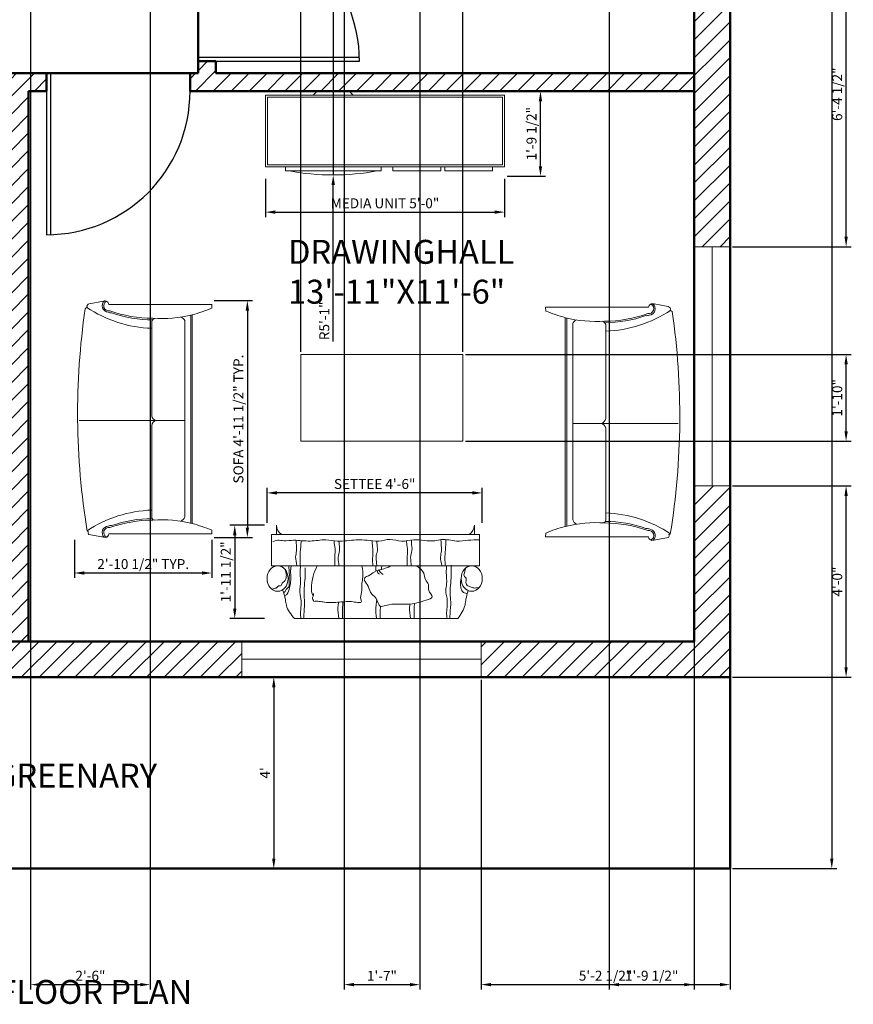
# Model space of a CAD drawing. Units: inches. Extents: x 3887 to 4286, y 884 to 1458.
# Tile 2 of 4: x 4077 to 4286, y 884 to 1131. Entities that reach past the tile are written whole.
import ezdxf

# ---------------------------------------------------------------- set-up
doc = ezdxf.new("R2010")
doc.units = ezdxf.units.IN
for name, color, linetype, lineweight in [('A-ANNO-DIMS', 2, 'Continuous', 18), ('A-ANNO-TEXT', 7, 'Continuous', 25), ('A-AREA-IDEN', 7, 'Continuous', 25), ('A-DOOR', 3, 'Continuous', 25), ('A-FURN', 8, 'Continuous', 18), ('A-GLAZ', 4, 'Continuous', 18), ('A-WALL', 7, 'Continuous', 50), ('A-WALL-PATT', 252, 'Continuous', 13)]:
    doc.layers.add(name, color=color, linetype=linetype, lineweight=lineweight)
doc.styles.get("Standard").update_dxf_attribs({"font": 'arial.ttf'})
doc.dimstyles.new('ISO-25', dxfattribs={"dimtxt": 2.5, "dimasz": 2.5, "dimexe": 1.25, "dimexo": 0.625, "dimtad": 1, "dimdec": 0, "dimlunit": 3, "dimtxsty": 'Standard', "dimcen": 2.5, "dimadec": 0, "dimazin": 0, "dimtfac": 1, "dimtdec": 0, "dimtmove": 0, "dimatfit": 3, "dimfxl": 1, "dimarcsym": 0})

# ---------------------------------------------------------------- blocks, each defined once
blk = doc.blocks.new('A$C69644375')
for p, q in [((1847.6, 919.1), (239.3, 919.1)), ((27.1, 91.8), (27.1, 399)), ((2073.7, 399), (27.1, 399)), ((2073.7, 399), (2073.7, 91.8)), ((2073.7, 91.8), (27.1, 91.8)), ((78.1, 91.8), (78.1, 0)), ((2025.4, 91.8), (2025.4, 0))]:
    blk.add_line(p, q)
for centre, start, end in [((187.1, -0.8), 121.46958, 179.57872), ((1916.5, -0.8), 0.42128, 58.53042)]:
    blk.add_arc(centre, 109, start, end)
at = {"extrusion": (0, 0, -1)}
for centre in [(103.9, 524.8), (2014.8, 524.8)]:
    blk.add_ellipse(centre, major_axis=(0, 125.7), ratio=0.82705, start_param=3.141593, end_param=9.424778, dxfattribs=at)
for points, knots in [([(137.7, 643.7), (147.1, 671.6), (161.1, 717.2), (170.9, 816.6), (209.4, 875.9), (239.3, 919.1)], [21.621392, 21.621392, 21.621392, 21.621392, 109.715225, 164.717522, 317.924576, 317.924576, 317.924576, 317.924576]), ([(318.6, 917.6), (317.6, 889.5), (316, 841.4), (307.9, 766.7), (315.9, 694.6), (316.1, 610.2), (302.9, 510.5), (305.2, 435.5), (306.5, 392.7)], [0, 0, 0, 0, 84.237495, 144.472456, 224.70795, 300.836536, 397.332321, 525.548945, 525.548945, 525.548945, 525.548945]), ([(346.9, 919.1), (349.1, 898.5), (352.8, 861.9), (344.6, 797.5), (341.7, 724.7), (365.6, 649.2), (342.5, 562.7), (358.6, 480.7), (352.8, 419.4), (350.6, 396.7)], [2.477757, 2.477757, 2.477757, 2.477757, 64.233403, 112.481299, 196.623447, 281.619849, 342.25328, 458.518645, 526.75141, 526.75141, 526.75141, 526.75141]), ([(671.2, 917.6), (671.9, 886.8), (673.2, 837.4), (668.4, 788.2), (667.2, 769.6)], [0, 0, 0, 0, 92.15571, 148.118503, 148.118503, 148.118503, 148.118503]), ([(707.2, 917.6), (712.9, 880.1), (720.1, 832.7), (712.8, 785.9), (711.3, 776.2)], [0, 0, 0, 0, 112.475377, 141.942796, 141.942796, 141.942796, 141.942796]), ([(1003.7, 917.6), (1004.5, 886.8), (1005.5, 846.8), (1002.6, 807.1), (1001.9, 798)], [0, 0, 0, 0, 92.15571, 119.67693, 119.67693, 119.67693, 119.67693]), ([(1039.8, 917.6), (1045.5, 880.1), (1054.2, 822.3), (1040.4, 760.3), (1039.1, 735.1), (1038.9, 730)], [0, 0, 0, 0, 112.475377, 173.108808, 188.403296, 188.403296, 188.403296, 188.403296]), ([(1376.3, 917.6), (1377.1, 886.8), (1378.5, 832.2), (1372.6, 777.9), (1371.6, 754.1)], [0, 0, 0, 0, 92.15571, 163.700074, 163.700074, 163.700074, 163.700074]), ([(1412.4, 917.6), (1418.1, 880.1), (1426.2, 826.7), (1415.9, 773.9), (1413.8, 758.1)], [0, 0, 0, 0, 112.475377, 160.127407, 160.127407, 160.127407, 160.127407]), ([(1757, 917.6), (1756.1, 889.5), (1754.5, 841.4), (1746.4, 766.7), (1754.3, 694.6), (1754.6, 610.2), (1742.2, 519.8), (1744, 454.1), (1745, 420.7)], [0, 0, 0, 0, 84.237495, 144.472456, 224.70795, 300.836536, 397.332321, 497.501547, 497.501547, 497.501547, 497.501547]), ([(1785.3, 919.1), (1787.5, 898.5), (1791.2, 861.9), (1783, 797.5), (1780.1, 724.7), (1804.1, 649.2), (1780.9, 562.7), (1797, 482), (1791.1, 422), (1789, 400.7)], [2.477757, 2.477757, 2.477757, 2.477757, 64.233403, 112.481299, 196.623447, 281.619849, 342.25328, 458.518645, 522.751997, 522.751997, 522.751997, 522.751997]), ([(1965.1, 635.2), (1954, 667.2), (1937.6, 716.7), (1928.4, 821.8), (1882.5, 878), (1847.6, 919.1)], [8.444588, 8.444588, 8.444588, 8.444588, 109.715225, 164.717522, 319.974725, 319.974725, 319.974725, 319.974725]), ([(1164, 540.9), (1149.2, 559.9), (1117.1, 601.1), (1100.8, 678.6), (1029.2, 716.5), (1023.2, 814.8), (886.4, 762.4), (735.7, 792.7), (603.6, 754.7), (466.8, 709.8), (540.8, 647.1), (520.4, 581.6), (567.2, 534.8), (568.3, 454.9), (616.9, 421.5), (647.1, 400.7)], [0, 0, 0, 0, 72.233047, 156.470492, 218.801185, 304.830125, 357.530882, 582.231345, 763.024758, 827.63193, 899.307199, 955.544862, 1014.704082, 1076.905882, 1178.90147, 1178.90147, 1178.90147, 1178.90147]), ([(1656.8, 749.3), (1639.4, 748.5), (1604.4, 747), (1521.3, 765.5), (1410.9, 759.8), (1291.1, 744.1), (1228, 763.8), (1183.4, 759.1), (1207.7, 711.2), (1178.9, 657), (1189.1, 581.5), (1169.4, 496.1), (1178.3, 438.3), (1184, 400.7)], [0, 0, 0, 0, 52.087932, 104.788603, 253.038902, 385.322741, 449.929867, 466.450206, 494.782313, 563.367144, 651.607113, 712.240498, 824.715876, 824.715876, 824.715876, 824.715876]), ([(1624.8, 400.7), (1639.9, 432.9), (1672.6, 502.7), (1682.2, 608.8), (1680.5, 659), (1668.8, 693.2), (1666.1, 685.2), (1664.8, 681.2)], [0, 0, 0, 0, 107.885542, 233.125089, 289.789384, 298.748781, 307.708142, 307.708142, 307.708142, 307.708142]), ([(1656.8, 749.3), (1664.8, 737.1), (1678.8, 715.8), (1659.5, 691.2), (1660.6, 677.2), (1660.9, 673)], [0, 0, 0, 0, 38.983085, 68.164145, 80.629677, 80.629677, 80.629677, 80.629677]), ([(1944.6, 700.6), (1937.4, 694.7), (1913.3, 671.5), (1899.8, 624.7), (1885.6, 565.8), (1884, 504.8), (1888.2, 447.1), (1882.7, 414), (1881.2, 404.7)], [34.701734, 34.701734, 34.701734, 34.701734, 62.587656, 136.251197, 173.191811, 245.424854, 317.546682, 345.878835, 345.878835, 345.878835, 345.878835]), ([(40, 613), (55.1, 616.5), (81.9, 622.6), (114.8, 602.8), (156.8, 597.6), (164, 555), (153.4, 520), (185.1, 504.2), (175.7, 465.1), (168.2, 441.4), (164.2, 428.7)], [0, 0, 0, 0, 44.256189, 78.489965, 112.723816, 158.407978, 186.455377, 209.121029, 245.181943, 287.01386, 287.01386, 287.01386, 287.01386]), ([(147.5, 674.2), (160.5, 671.6), (192.4, 665.4), (222.4, 596), (211.6, 543), (204.5, 508)], [0, 0, 0, 0, 38.011492, 93.00469, 199.417844, 199.417844, 199.417844, 199.417844]), ([(1955.3, 664.3), (1949.7, 661.6), (1936.7, 652), (1931.5, 625), (1901, 612.3), (1902, 536.8), (1895.8, 472.8), (1903.7, 415.4), (1905.2, 404.7)], [33.002736, 33.002736, 33.002736, 33.002736, 52.087989, 84.391566, 104.42539, 141.366005, 281.602903, 313.906504, 313.906504, 313.906504, 313.906504]), ([(2061.5, 621), (2046.3, 621.9), (2022.8, 623.2), (2009, 591.4), (1977.1, 604.2), (1975, 565.6), (1937.3, 551.2), (1929.2, 512.4), (1928.2, 473.5), (1936, 454), (1941.3, 440.7)], [0, 0, 0, 0, 40.861148, 63.526857, 83.56064, 115.864217, 141.52001, 197.327846, 217.361728, 259.193601, 259.193601, 259.193601, 259.193601]), ([(1160, 532.9), (1159.2, 527.1), (1156.4, 506.9), (1107.3, 497.5), (1058.9, 447.6), (977.8, 435.3), (923.1, 412.5), (900, 401), (896.2, 399)], [0, 0, 0, 0, 16.520339, 57.77249, 124.458333, 225.822378, 290.553607, 303.2098, 303.2098, 303.2098, 303.2098]), ([(1019.7, 436.7), (1016.1, 443.7), (1005.7, 463.3), (987.4, 476.4), (975.7, 484.8)], [0, 0, 0, 0, 23.363259, 65.955745, 65.955745, 65.955745, 65.955745]), ([(364.3, 399), (365.1, 387.6), (368, 350.7), (368.2, 281.6), (358.1, 207.4), (357.5, 158.2), (357.6, 141)], [190.255604, 190.255604, 190.255604, 190.255604, 224.70795, 300.836536, 397.332321, 448.655162, 448.655162, 448.655162, 448.655162]), ([(398.4, 399), (398.5, 398.3), (402.3, 369.2), (417.8, 320.6), (394.6, 235.6), (407, 177.9), (406.8, 140.7)], [194.236029, 194.236029, 194.236029, 194.236029, 196.623447, 281.619849, 342.25328, 454.038772, 454.038772, 454.038772, 454.038772]), ([(698.2, 399), (698.3, 392.9), (700.2, 358.5), (711.7, 313.8), (687.5, 252.5), (694.1, 201.4), (698.1, 160.3), (698.2, 146.5)], [190.129367, 190.129367, 190.129367, 190.129367, 208.421077, 292.658572, 321.828316, 401.96366, 443.368776, 443.368776, 443.368776, 443.368776]), ([(738.4, 399), (737.9, 374.3), (742.3, 323.9), (730.9, 250.8), (742.4, 194.1), (745.1, 162.4), (745.6, 153.4)], [190.836968, 190.836968, 190.836968, 190.836968, 265.264473, 341.498474, 410.083305, 437.099432, 437.099432, 437.099432, 437.099432]), ([(1031.8, 448.8), (1031.5, 456.1), (1030.9, 470.6), (1018.1, 477.4), (1011.7, 480.8)], [0, 0, 0, 0, 20.430573, 40.464424, 40.464424, 40.464424, 40.464424]), ([(1038.7, 399), (1038.9, 392.9), (1040.7, 358.5), (1052.2, 313.8), (1028.1, 252.5), (1034.2, 205), (1037.9, 167.4), (1038.5, 157)], [190.129367, 190.129367, 190.129367, 190.129367, 208.421077, 292.658572, 321.828316, 401.96366, 432.870883, 432.870883, 432.870883, 432.870883]), ([(1078.9, 399), (1078.4, 374.3), (1082.9, 323.9), (1071.4, 250.8), (1082.9, 194.3), (1085.6, 162.7), (1086.2, 153.9)], [190.836968, 190.836968, 190.836968, 190.836968, 265.264473, 341.498474, 410.083305, 436.597925, 436.597925, 436.597925, 436.597925]), ([(1411.4, 399), (1411.5, 392.9), (1413.4, 358.5), (1424.9, 313.8), (1400.7, 252.5), (1406.8, 204.9), (1410.6, 167.2), (1411.1, 156.8)], [190.129367, 190.129367, 190.129367, 190.129367, 208.421077, 292.658572, 321.828316, 401.96366, 433.110807, 433.110807, 433.110807, 433.110807]), ([(1451.6, 399), (1451.1, 374.3), (1455.5, 323.9), (1444.1, 250.8), (1455.6, 194), (1458.3, 162.1), (1458.9, 152.9)], [190.836968, 190.836968, 190.836968, 190.836968, 265.264473, 341.498474, 410.083305, 437.573854, 437.573854, 437.573854, 437.573854]), ([(1790.7, 399), (1791.5, 387.6), (1794.4, 350.7), (1794.6, 281.6), (1785, 210.8), (1784, 165.1), (1784, 151.4)], [190.255604, 190.255604, 190.255604, 190.255604, 224.70795, 300.836536, 397.332321, 438.291577, 438.291577, 438.291577, 438.291577]), ([(1824.8, 399), (1824.9, 398.3), (1828.7, 369.2), (1844.2, 320.6), (1821.7, 238.2), (1832.4, 183), (1833.1, 148.3)], [194.236029, 194.236029, 194.236029, 194.236029, 196.623447, 281.619849, 342.25328, 446.449161, 446.449161, 446.449161, 446.449161]), ([(2061.5, 160.3), (2045.6, 154.9), (2010.3, 143.1), (1941.1, 157.7), (1834.5, 140.2), (1696.7, 167.9), (1552.4, 133.8), (1402, 167.9), (1265.6, 139.7), (1130.5, 145.9), (1019.2, 166.3), (907.6, 126.7), (793, 169.1), (646.4, 126.8), (513.3, 169.9), (375.5, 127.4), (265.2, 167.3), (141, 145.4), (66.1, 144.6), (30.1, 144.2)], [0, 0, 0, 0, 49.560916, 109.795839, 206.041565, 370.514196, 523.244954, 640.061112, 824.76374, 933.020566, 1045.495763, 1158.824136, 1272.152508, 1392.954889, 1601.460588, 1666.685979, 1815.800011, 1932.272164, 2040.52891, 2040.52891, 2040.52891, 2040.52891])]:
    blk.add_open_spline(points, degree=3, knots=knots)
for points in [[(995.1, 436.3), (993.3, 423), (990.5, 409.8), (987.7, 396.7)], [(1047.5, 452.6), (1047.9, 435.3), (1047.9, 418), (1047.8, 400.7)]]:
    blk.add_open_spline(points, degree=3)
blk = doc.blocks.new('A$C73531C16')
for p, q in [((797.3, 883), (797.3, 180.7)), ((797.3, 883), (797.3, 180.7)), ((19.2, 817.1), (1.4, 722.3)), ((19.2, 817.1), (1.4, 722.3)), ((1533.5, 830.9), (1538.9, 821.6)), ((1533.5, 830.9), (1538.9, 821.6)), ((1576, 707.8), (1556.2, 818.7)), ((1576, 707.8), (1556.2, 818.7)), ((23.8, 686), (23.8, 0)), ((23.8, 686), (23.8, 0)), ((1552.7, 686), (1552.7, 0)), ((1552.7, 686), (1552.7, 0)), ((137.5, 400.7), (765.2, 400.7)), ((137.5, 400.7), (765.2, 400.7)), ((829.2, 400.7), (1440.8, 400.7)), ((829.2, 400.7), (1440.8, 400.7)), ((93.7, 140.7), (1483.4, 140.7)), ((93.7, 140.7), (1483.4, 140.7)), ((132, 180.7), (1440.1, 180.7)), ((132, 180.7), (1440.1, 180.7)), ((93, 130.7), (1483.4, 130.7)), ((93, 130.7), (1483.4, 130.7)), ((23.8, 0), (48.7, 0.9)), ((23.8, 0), (48.7, 0.9)), ((1527.8, 0.9), (1552.7, 0)), ((1527.8, 0.9), (1552.7, 0))]:
    blk.add_line(p, q)
for centre, radius, start, end in [((750, -3986.3), 4880.5, 80.76194, 98.21709), ((750, -3986.3), 4880.5, 80.76194, 98.21709), ((37, 813.7), 18.2, 70.94115, 169.10122), ((37, 813.7), 18.2, 70.94115, 169.10122), ((151.8, 763), 128.2, 140.79379, 148.04958), ((151.8, 763), 128.2, 140.79379, 148.04958), ((-655.1, 369.6), 838.8, 2.12384, 33.52274), ((-655.1, 369.6), 838.8, 2.12384, 33.52274), ((2230.9, 369.6), 838.2, 146.55548, 177.87575), ((2230.9, 369.6), 838.2, 146.55548, 177.87575), ((1546.2, 809.1), 14.4, 42.1894, 120.22739), ((1546.2, 809.1), 14.4, 42.1894, 120.22739), ((27.6, 713.3), 27.6, 161.10495, 262.17796), ((27.6, 713.3), 27.6, 161.10495, 262.17796), ((33, 687), 43.5, 3.68024, 139.32094), ((33, 687), 43.5, 3.68024, 139.32094), ((1543.4, 687), 43.5, 45.07885, 176.31976), ((1543.4, 687), 43.5, 45.07885, 176.31976), ((33, 687), 33.5, 348.63115, 153.12764), ((33, 687), 33.5, 348.63115, 153.12764), ((-739.7, 390.8), 856.1, 0.18203, 19.77552), ((-739.7, 390.8), 856.1, 0.18203, 19.77552), ((41.2, 673.9), 38.7, 351.85588, 24.24722), ((41.2, 673.9), 38.7, 351.85588, 24.24722), ((-719.3, 390.7), 845.7, 0.16174, 19.17027), ((-719.3, 390.7), 845.7, 0.16174, 19.17027), ((2288, 392), 838, 160.74027, 179.53449), ((2288, 392), 838, 160.74027, 179.53449), ((2316.1, 390.8), 856.1, 160.22448, 179.81797), ((2316.1, 390.8), 856.1, 160.22448, 179.81797), ((1535.3, 673.9), 38.7, 155.75278, 188.14412), ((1535.3, 673.9), 38.7, 155.75278, 188.14412), ((1543.4, 687), 33.5, 26.87236, 191.36885), ((1543.4, 687), 33.5, 26.87236, 191.36885), ((1548.9, 713.3), 27.6, 277.82204, 348.41793), ((1548.9, 713.3), 27.6, 277.82204, 348.41793), ((-717.7, 335.2), 836.1, 345.84723, 4.00033), ((-717.7, 335.2), 836.1, 345.84723, 4.00033), ((156.6, 360.6), 44.4, 115.39182, 154.20701), ((156.6, 360.6), 44.4, 115.39182, 154.20701), ((756.8, 359.5), 42, 16.04192, 78.50349), ((756.8, 359.5), 42, 16.04192, 78.50349), ((837.6, 359.5), 42, 101.49651, 163.95808), ((837.6, 359.5), 42, 101.49651, 163.95808), ((1442.2, 383.3), 17.5, 3.33645, 94.38408), ((1442.2, 383.3), 17.5, 3.33645, 94.38408), ((2294.2, 335.2), 836.1, 175.99967, 194.15277), ((2294.2, 335.2), 836.1, 175.99967, 194.15277), ((149.3, 221.6), 44.4, 202.02539, 247.09465), ((149.3, 221.6), 44.4, 202.02539, 247.09465), ((1425.5, 222.6), 44.4, 289.11707, 341.80542), ((1425.5, 222.6), 44.4, 289.11707, 341.80542), ((-1077.6, 458.1), 1215.5, 337.90453, 344.37633), ((-1077.6, 458.1), 1215.5, 337.90453, 344.37633), ((2285.2, 332.1), 826.6, 194.09858, 203.62056), ((2285.2, 332.1), 826.6, 194.09858, 203.62056)]:
    blk.add_arc(centre, radius, start, end)
blk = doc.blocks.new('A$C4B5722C8')
blk.add_blockref('A$C73531C16', (0, 0))
blk = doc.blocks.new('Entertainment Center')
for p, q in [((-4, 0), (-5, -1)), ((4, 0), (-4, 0)), ((5, -1), (4, 0)), ((-17, -19), (-17, -1)), ((-17, -1), (43, -1)), ((-16.5, -18.5), (-16.5, -1.5)), ((-16.5, -1.5), (42.5, -1.5)), ((42.5, -1.5), (42.5, -18.5)), ((43, -1), (43, -19)), ((43, -19), (-17, -19)), ((42.5, -18.5), (-16.5, -18.5)), ((-12, -20), (-12, -19)), ((12, -19), (12, -20)), ((15, -20), (15, -19)), ((27, -19), (27, -20)), ((28, -20), (28, -19)), ((40, -19), (40, -20)), ((12, -20), (-12, -20)), ((27, -20), (15, -20)), ((40, -20), (28, -20))]:
    blk.add_line(p, q)
blk.add_arc((0, 40), 61, 259.6111, 280.3889)
blk = doc.blocks.new('*D9')
at = {"layer": 'A-ANNO-DIMS', "color": 0, "lineweight": -2, "transparency": 16777216}
for p, q in [((4150.96, 965.64), (4139.44, 965.64)), ((4140.69, 963.14), (4140.69, 920.14)), ((4150.96, 917.64), (4139.44, 917.64))]:
    blk.add_line(p, q, dxfattribs=at)
at = {"layer": 'A-ANNO-DIMS', "color": 0, "transparency": 16777216}
for points in [[(4140.27, 963.14), (4141.11, 963.14), (4140.69, 965.64)], [(4140.27, 920.14), (4141.11, 920.14), (4140.69, 917.64)]]:
    blk.add_solid(points, dxfattribs=at)
at = {"layer": 'Defpoints', "color": 0, "transparency": 16777216}
for p in [(4151.58, 965.64), (4140.69, 917.64), (4151.58, 917.64)]:
    blk.add_point(p, dxfattribs=at)
at = {"layer": 'A-ANNO-DIMS', "color": 0, "transparency": 16777216, "insert": (4138.82, 941.64), "char_height": 2.5, "attachment_point": 5, "rotation": 90}
blk.add_mtext("4'", dxfattribs=at)
blk = doc.blocks.new('*D11')
at = {"layer": 'A-ANNO-DIMS', "color": 0, "lineweight": -2, "transparency": 16777216}
for p, q in [((4255.81, 1394.64), (4281.94, 1394.64)), ((4280.69, 1392.14), (4280.69, 920.14)), ((4255.81, 917.64), (4281.94, 917.64))]:
    blk.add_line(p, q, dxfattribs=at)
at = {"layer": 'A-ANNO-DIMS', "color": 0, "transparency": 16777216}
for points in [[(4280.27, 1392.14), (4281.11, 1392.14), (4280.69, 1394.64)], [(4280.27, 920.14), (4281.11, 920.14), (4280.69, 917.64)]]:
    blk.add_solid(points, dxfattribs=at)
at = {"layer": 'Defpoints', "color": 0, "transparency": 16777216}
for p in [(4255.18, 1394.64), (4255.18, 917.64), (4280.69, 917.64)]:
    blk.add_point(p, dxfattribs=at)
at = {"layer": 'A-ANNO-DIMS', "color": 0, "transparency": 16777216, "insert": (4278.79, 1156.14), "char_height": 2.5, "attachment_point": 5, "rotation": 90}
blk.add_mtext('39\'-9"', dxfattribs=at)
blk = doc.blocks.new('DOOR-SWING-36IN')
for p, q in [((35, 0), (35, 40.5)), ((36, 4.5), (36, 40.5))]:
    blk.add_line(p, q)
blk.add_arc((36, 4.5), 36, 90, 180)
blk = doc.blocks.new('WIN-GLAZ-60IN')
for p, q in [((60, 9), (0, 9)), ((0, 4.5), (60, 4.5)), ((0, 0), (60, 0))]:
    blk.add_line(p, q)
blk = doc.blocks.new('*D21')
at = {"layer": 'A-ANNO-DIMS', "color": 0, "lineweight": -2, "transparency": 16777216}
for p, q in [((4125.77, 1060.11), (4135.31, 1060.11)), ((4134.06, 1057.61), (4134.06, 1003.2)), ((4125.77, 1000.7), (4135.31, 1000.7))]:
    blk.add_line(p, q, dxfattribs=at)
at = {"layer": 'A-ANNO-DIMS', "color": 0, "transparency": 16777216}
for points in [[(4133.64, 1057.61), (4134.48, 1057.61), (4134.06, 1060.11)], [(4133.64, 1003.2), (4134.48, 1003.2), (4134.06, 1000.7)]]:
    blk.add_solid(points, dxfattribs=at)
at = {"layer": 'Defpoints', "color": 0, "transparency": 16777216}
for p in [(4125.15, 1060.11), (4125.15, 1000.7), (4134.06, 1000.7)]:
    blk.add_point(p, dxfattribs=at)
at = {"layer": 'A-ANNO-DIMS', "color": 0, "transparency": 16777216, "insert": (4132.14, 1030.41), "char_height": 2.5, "attachment_point": 5, "rotation": 90}
blk.add_mtext('SOFA 4\'-11 1/2" TYP.', dxfattribs=at)
blk = doc.blocks.new('*D22')
at = {"layer": 'A-ANNO-DIMS', "color": 0, "lineweight": -2, "transparency": 16777216}
for p, q in [((4090.68, 1000.08), (4090.68, 990.54)), ((4125.15, 1000.08), (4125.15, 990.54)), ((4122.65, 991.79), (4093.18, 991.79))]:
    blk.add_line(p, q, dxfattribs=at)
at = {"layer": 'A-ANNO-DIMS', "color": 0, "transparency": 16777216}
for points in [[(4093.18, 992.21), (4093.18, 991.37), (4090.68, 991.79)], [(4122.65, 992.21), (4122.65, 991.37), (4125.15, 991.79)]]:
    blk.add_solid(points, dxfattribs=at)
at = {"layer": 'Defpoints', "color": 0, "transparency": 16777216}
for p in [(4090.68, 1000.7), (4125.15, 1000.7), (4090.68, 991.79)]:
    blk.add_point(p, dxfattribs=at)
at = {"layer": 'A-ANNO-DIMS', "color": 0, "transparency": 16777216, "insert": (4107.92, 993.71), "char_height": 2.5, "attachment_point": 5}
blk.add_mtext('2\'-10 1/2" TYP.', dxfattribs=at)
blk = doc.blocks.new('*D27')
at = {"layer": 'A-ANNO-DIMS', "color": 0, "lineweight": -2, "transparency": 16777216}
for p, q in [((4138.99, 1004.41), (4138.99, 1013.14)), ((4193, 1004.41), (4193, 1013.14)), ((4190.5, 1011.89), (4141.49, 1011.89))]:
    blk.add_line(p, q, dxfattribs=at)
at = {"layer": 'A-ANNO-DIMS', "color": 0, "transparency": 16777216}
for points in [[(4141.49, 1012.3), (4141.49, 1011.47), (4138.99, 1011.89)], [(4190.5, 1012.3), (4190.5, 1011.47), (4193, 1011.89)]]:
    blk.add_solid(points, dxfattribs=at)
at = {"layer": 'Defpoints', "color": 0, "transparency": 16777216}
for p in [(4138.99, 1011.89), (4138.99, 1003.78), (4193, 1003.78)]:
    blk.add_point(p, dxfattribs=at)
at = {"layer": 'A-ANNO-DIMS', "color": 0, "transparency": 16777216, "insert": (4166, 1013.8), "char_height": 2.5, "attachment_point": 5}
blk.add_mtext('SETTEE 4\'-6"', dxfattribs=at)
blk = doc.blocks.new('*D28')
at = {"layer": 'A-ANNO-DIMS', "color": 0, "lineweight": -2, "transparency": 16777216}
for p, q in [((4138.37, 1003.78), (4129.64, 1003.78)), ((4130.89, 1001.28), (4130.89, 982.86)), ((4138.37, 980.36), (4129.64, 980.36))]:
    blk.add_line(p, q, dxfattribs=at)
at = {"layer": 'A-ANNO-DIMS', "color": 0, "transparency": 16777216}
for points in [[(4130.48, 1001.28), (4131.31, 1001.28), (4130.89, 1003.78)], [(4130.48, 982.86), (4131.31, 982.86), (4130.89, 980.36)]]:
    blk.add_solid(points, dxfattribs=at)
at = {"layer": 'Defpoints', "color": 0, "transparency": 16777216}
for p in [(4138.99, 1003.78), (4130.89, 980.36), (4138.99, 980.36)]:
    blk.add_point(p, dxfattribs=at)
at = {"layer": 'A-ANNO-DIMS', "color": 0, "transparency": 16777216, "insert": (4128.98, 992.07), "char_height": 2.5, "attachment_point": 5, "rotation": 90}
blk.add_mtext('1\'-11 1/2"', dxfattribs=at)
blk = doc.blocks.new('*D29')
at = {"layer": 'A-ANNO-DIMS', "color": 0, "lineweight": -2, "transparency": 16777216}
for p, q in [((4138.6, 1090.69), (4138.6, 1081.06)), ((4198.6, 1090.69), (4198.6, 1081.06)), ((4141.1, 1082.31), (4196.1, 1082.31))]:
    blk.add_line(p, q, dxfattribs=at)
at = {"layer": 'A-ANNO-DIMS', "color": 0, "transparency": 16777216}
for points in [[(4141.1, 1082.73), (4141.1, 1081.89), (4138.6, 1082.31)], [(4196.1, 1082.73), (4196.1, 1081.89), (4198.6, 1082.31)]]:
    blk.add_solid(points, dxfattribs=at)
at = {"layer": 'Defpoints', "color": 0, "transparency": 16777216}
for p in [(4138.6, 1091.31), (4198.6, 1091.31), (4198.6, 1082.31)]:
    blk.add_point(p, dxfattribs=at)
at = {"layer": 'A-ANNO-DIMS', "color": 0, "transparency": 16777216, "insert": (4168.6, 1084.21), "char_height": 2.5, "attachment_point": 5}
blk.add_mtext('MEDIA UNIT 5\'-0"', dxfattribs=at)
blk = doc.blocks.new('*D30')
at = {"layer": 'A-ANNO-DIMS', "color": 0, "lineweight": -2, "transparency": 16777216}
for p, q in [((4199.22, 1112.64), (4208.85, 1112.64)), ((4207.6, 1093.81), (4207.6, 1110.14)), ((4199.22, 1091.31), (4208.85, 1091.31))]:
    blk.add_line(p, q, dxfattribs=at)
at = {"layer": 'A-ANNO-DIMS', "color": 0, "transparency": 16777216}
for points in [[(4207.18, 1110.14), (4208.01, 1110.14), (4207.6, 1112.64)], [(4207.18, 1093.81), (4208.01, 1093.81), (4207.6, 1091.31)]]:
    blk.add_solid(points, dxfattribs=at)
at = {"layer": 'Defpoints', "color": 0, "transparency": 16777216}
for p in [(4198.6, 1112.64), (4207.6, 1112.64), (4198.6, 1091.31)]:
    blk.add_point(p, dxfattribs=at)
at = {"layer": 'A-ANNO-DIMS', "color": 0, "transparency": 16777216, "insert": (4205.68, 1101.98), "char_height": 2.5, "attachment_point": 5, "rotation": 90}
blk.add_mtext('1\'-9 1/2"', dxfattribs=at)
blk = doc.blocks.new('*D33')
at = {"layer": 'A-ANNO-DIMS', "color": 0, "lineweight": -2, "transparency": 16777216}
for p, q in [((4255.81, 1013.64), (4285.53, 1013.64)), ((4284.28, 968.14), (4284.28, 1011.14)), ((4255.81, 965.64), (4285.53, 965.64))]:
    blk.add_line(p, q, dxfattribs=at)
at = {"layer": 'A-ANNO-DIMS', "color": 0, "transparency": 16777216}
for points in [[(4283.87, 1011.14), (4284.7, 1011.14), (4284.28, 1013.64)], [(4283.87, 968.14), (4284.7, 968.14), (4284.28, 965.64)]]:
    blk.add_solid(points, dxfattribs=at)
at = {"layer": 'Defpoints', "color": 0, "transparency": 16777216}
for p in [(4255.18, 1013.64), (4284.28, 1013.64), (4255.18, 965.64)]:
    blk.add_point(p, dxfattribs=at)
at = {"layer": 'A-ANNO-DIMS', "color": 0, "transparency": 16777216, "insert": (4282.38, 989.64), "char_height": 2.5, "attachment_point": 5, "rotation": 90}
blk.add_mtext('4\'-0"', dxfattribs=at)
blk = doc.blocks.new('*D34')
at = {"layer": 'A-ANNO-DIMS', "color": 0, "lineweight": -2, "transparency": 16777216}
for p, q in [((4255.81, 1150.14), (4285.53, 1150.14)), ((4284.28, 1076.14), (4284.28, 1147.64)), ((4255.81, 1073.64), (4285.53, 1073.64))]:
    blk.add_line(p, q, dxfattribs=at)
at = {"layer": 'A-ANNO-DIMS', "color": 0, "transparency": 16777216}
for points in [[(4283.87, 1147.64), (4284.7, 1147.64), (4284.28, 1150.14)], [(4283.87, 1076.14), (4284.7, 1076.14), (4284.28, 1073.64)]]:
    blk.add_solid(points, dxfattribs=at)
at = {"layer": 'Defpoints', "color": 0, "transparency": 16777216}
for p in [(4255.18, 1150.14), (4284.28, 1150.14), (4255.18, 1073.64)]:
    blk.add_point(p, dxfattribs=at)
at = {"layer": 'A-ANNO-DIMS', "color": 0, "transparency": 16777216, "insert": (4282.37, 1111.89), "char_height": 2.5, "attachment_point": 5, "rotation": 90}
blk.add_mtext('6\'-4 1/2"', dxfattribs=at)
blk = doc.blocks.new('*D42')
at = {"layer": 'A-ANNO-DIMS', "color": 0, "lineweight": -2, "transparency": 16777216}
for p, q in [((4192.68, 965.02), (4192.68, 887.29)), ((4255.18, 965.02), (4255.18, 887.29)), ((4195.18, 888.54), (4252.68, 888.54))]:
    blk.add_line(p, q, dxfattribs=at)
at = {"layer": 'A-ANNO-DIMS', "color": 0, "transparency": 16777216}
for points in [[(4195.18, 888.96), (4195.18, 888.13), (4192.68, 888.54)], [(4252.68, 888.96), (4252.68, 888.13), (4255.18, 888.54)]]:
    blk.add_solid(points, dxfattribs=at)
at = {"layer": 'Defpoints', "color": 0, "transparency": 16777216}
for p in [(4192.68, 965.64), (4255.18, 965.64), (4255.18, 888.54)]:
    blk.add_point(p, dxfattribs=at)
at = {"layer": 'A-ANNO-DIMS', "color": 0, "transparency": 16777216, "insert": (4223.93, 890.46), "char_height": 2.5, "attachment_point": 5}
blk.add_mtext('5\'-2 1/2"', dxfattribs=at)
blk = doc.blocks.new('*D48')
at = {"layer": 'A-ANNO-DIMS', "color": 0, "lineweight": -2, "transparency": 16777216}
for p, q in [((4147.49, 1047.25), (4147.49, 1424.99)), ((4149.99, 1423.74), (4185.63, 1423.74)), ((4188.13, 1047.25), (4188.13, 1424.99))]:
    blk.add_line(p, q, dxfattribs=at)
at = {"layer": 'A-ANNO-DIMS', "color": 0, "transparency": 16777216}
for points in [[(4149.99, 1424.16), (4149.99, 1423.33), (4147.49, 1423.74)], [(4185.63, 1424.16), (4185.63, 1423.33), (4188.13, 1423.74)]]:
    blk.add_solid(points, dxfattribs=at)
at = {"layer": 'Defpoints', "color": 0, "transparency": 16777216}
for p in [(4188.13, 1423.74), (4147.49, 1046.63), (4188.13, 1046.63)]:
    blk.add_point(p, dxfattribs=at)
at = {"layer": 'A-ANNO-DIMS', "color": 0, "transparency": 16777216, "insert": (4167.81, 1425.66), "char_height": 2.5, "attachment_point": 5}
blk.add_mtext('3\'-4 1/2"', dxfattribs=at)
blk = doc.blocks.new('*D49')
at = {"layer": 'A-ANNO-DIMS', "color": 0, "lineweight": -2, "transparency": 16777216}
for p, q in [((4188.76, 1046.63), (4285.53, 1046.63)), ((4284.28, 1027.33), (4284.28, 1044.13)), ((4188.76, 1024.83), (4285.53, 1024.83))]:
    blk.add_line(p, q, dxfattribs=at)
at = {"layer": 'A-ANNO-DIMS', "color": 0, "transparency": 16777216}
for points in [[(4283.87, 1044.13), (4284.7, 1044.13), (4284.28, 1046.63)], [(4283.87, 1027.33), (4284.7, 1027.33), (4284.28, 1024.83)]]:
    blk.add_solid(points, dxfattribs=at)
at = {"layer": 'Defpoints', "color": 0, "transparency": 16777216}
for p in [(4188.13, 1046.63), (4284.28, 1046.63), (4188.13, 1024.83)]:
    blk.add_point(p, dxfattribs=at)
at = {"layer": 'A-ANNO-DIMS', "color": 0, "transparency": 16777216, "insert": (4282.38, 1035.73), "char_height": 2.5, "attachment_point": 5, "rotation": 90}
blk.add_mtext('1\'-10"', dxfattribs=at)
blk = doc.blocks.new('*D50')
at = {"layer": 'A-ANNO-DIMS', "color": 0, "lineweight": -2, "transparency": 16777216}
for p, q in [((4224.82, 1283.02), (4224.82, 887.29)), ((4246.18, 1283.02), (4246.18, 887.29)), ((4227.32, 888.54), (4243.68, 888.54))]:
    blk.add_line(p, q, dxfattribs=at)
at = {"layer": 'A-ANNO-DIMS', "color": 0, "transparency": 16777216}
for points in [[(4227.32, 888.96), (4227.32, 888.13), (4224.82, 888.54)], [(4243.68, 888.96), (4243.68, 888.13), (4246.18, 888.54)]]:
    blk.add_solid(points, dxfattribs=at)
at = {"layer": 'Defpoints', "color": 0, "transparency": 16777216}
for p in [(4224.82, 1283.64), (4246.18, 1283.64), (4246.18, 888.54)]:
    blk.add_point(p, dxfattribs=at)
at = {"layer": 'A-ANNO-DIMS', "color": 0, "transparency": 16777216, "insert": (4235.5, 890.46), "char_height": 2.5, "attachment_point": 5}
blk.add_mtext('1\'-9 1/2"', dxfattribs=at)
blk = doc.blocks.new('*D54')
at = {"layer": 'A-ANNO-DIMS', "color": 0, "lineweight": -2, "transparency": 16777216}
for p, q in [((4158.31, 1372.33), (4158.31, 887.29)), ((4177.34, 1372.33), (4177.34, 887.29)), ((4160.81, 888.54), (4174.84, 888.54))]:
    blk.add_line(p, q, dxfattribs=at)
at = {"layer": 'A-ANNO-DIMS', "color": 0, "transparency": 16777216}
for points in [[(4160.81, 888.96), (4160.81, 888.13), (4158.31, 888.54)], [(4174.84, 888.96), (4174.84, 888.13), (4177.34, 888.54)]]:
    blk.add_solid(points, dxfattribs=at)
at = {"layer": 'Defpoints', "color": 0, "transparency": 16777216}
for p in [(4158.31, 1372.95), (4177.34, 1372.95), (4177.34, 888.54)]:
    blk.add_point(p, dxfattribs=at)
at = {"layer": 'A-ANNO-DIMS', "color": 0, "transparency": 16777216, "insert": (4167.82, 890.42), "char_height": 2.5, "attachment_point": 5}
blk.add_mtext('1\'-7"', dxfattribs=at)
blk = doc.blocks.new('*D59')
at = {"layer": 'A-ANNO-DIMS', "color": 0, "lineweight": -2, "transparency": 16777216}
for p, q in [((4079.68, 1290.52), (4079.68, 887.29)), ((4109.68, 1290.52), (4109.68, 887.29)), ((4082.18, 888.54), (4107.18, 888.54))]:
    blk.add_line(p, q, dxfattribs=at)
at = {"layer": 'A-ANNO-DIMS', "color": 0, "transparency": 16777216}
for points in [[(4082.18, 888.96), (4082.18, 888.13), (4079.68, 888.54)], [(4107.18, 888.96), (4107.18, 888.13), (4109.68, 888.54)]]:
    blk.add_solid(points, dxfattribs=at)
at = {"layer": 'Defpoints', "color": 0, "transparency": 16777216}
for p in [(4079.68, 1291.14), (4109.68, 1291.14), (4109.68, 888.54)]:
    blk.add_point(p, dxfattribs=at)
at = {"layer": 'A-ANNO-DIMS', "color": 0, "transparency": 16777216, "insert": (4094.68, 890.45), "char_height": 2.5, "attachment_point": 5}
blk.add_mtext('2\'-6"', dxfattribs=at)
blk = doc.blocks.new('*D60')
at = {"layer": 'A-ANNO-DIMS', "color": 0, "lineweight": -2, "transparency": 16777216}
for p, q in [((4155.6, 1152.64), (4155.6, 1091.64)), ((4155.6, 1049.9), (4155.6, 1089.14))]:
    blk.add_line(p, q, dxfattribs=at)
at = {"layer": 'A-ANNO-DIMS', "color": 0, "transparency": 16777216}
blk.add_solid([(4155.18, 1089.14), (4156.01, 1089.14), (4155.6, 1091.64)], dxfattribs=at)
at = {"layer": 'Defpoints', "color": 0, "transparency": 16777216}
for p in [(4155.6, 1152.64), (4155.6, 1091.64)]:
    blk.add_point(p, dxfattribs=at)
at = {"layer": 'A-ANNO-DIMS', "color": 0, "transparency": 16777216, "insert": (4153.7, 1055.04), "char_height": 2.5, "attachment_point": 5, "rotation": 90}
blk.add_mtext('R5\'-1"', dxfattribs=at)

msp = doc.modelspace()

# ---------------------------------------------------------------- hatches: boundary and pattern name
at = {"layer": 'A-WALL-PATT'}
h = msp.add_hatch(dxfattribs=at)
h.set_pattern_fill('ANSI31', color=256)
h.paths.add_polyline_path([(4079.68, 1394.64), (3922.18, 1394.64), (3922.18, 1343.64), (3931.18, 1343.64), (3931.18, 1385.64), (4079.68, 1385.64)])
h.paths.add_polyline_path([(4156.18, 1394.64), (4109.68, 1394.64), (4109.68, 1385.64), (4156.18, 1385.64)])
h.paths.add_polyline_path([(4255.18, 1394.64), (4216.18, 1394.64), (4216.18, 1385.64), (4246.18, 1385.64), (4246.18, 1343.64), (4255.18, 1343.64)])
h.paths.add_polyline_path([(3931.18, 1283.64), (3922.18, 1283.64), (3922.18, 1207.14), (3931.18, 1207.14)])
h.paths.add_polyline_path([(4024.18, 1241.64), (3931.18, 1241.64), (3931.18, 1237.14), (4024.18, 1237.14)])
h.paths.add_polyline_path([(4067.68, 1291.14), (4079.68, 1291.14), (4079.68, 1295.64), (4067.68, 1295.64), (4067.68, 1385.64), (4063.18, 1385.64), (4063.18, 1241.64), (4060.18, 1241.64), (4060.18, 1237.14), (4067.68, 1237.14)])
h.paths.add_polyline_path([(4126.18, 1385.64), (4121.68, 1385.64), (4121.68, 1295.64), (4109.68, 1295.64), (4109.68, 1291.14), (4121.68, 1291.14), (4121.68, 1280.64), (4126.18, 1280.64)])
h.paths.add_polyline_path([(4246.18, 1241.64), (4126.18, 1241.64), (4126.18, 1244.64), (4121.68, 1244.64), (4121.68, 1156.14), (4126.18, 1156.14), (4126.18, 1237.14), (4246.18, 1237.14)])
h.paths.add_polyline_path([(4255.18, 1283.64), (4246.18, 1283.64), (4246.18, 1210.14), (4255.18, 1210.14)])
h.paths.add_polyline_path([(4255.18, 1150.14), (4246.18, 1150.14), (4246.18, 1073.64), (4255.18, 1073.64)])
h.paths.add_polyline_path([(4246.18, 1117.14), (4126.18, 1117.14), (4126.18, 1120.14), (4121.68, 1120.14), (4121.68, 1117.14), (4119.68, 1117.14), (4119.68, 1112.64), (4246.18, 1112.64)])
h.paths.add_polyline_path([(4079.18, 1112.64), (4083.68, 1112.64), (4083.68, 1117.14), (4074.68, 1117.14), (4074.68, 974.64), (4079.18, 974.64)])
h.paths.add_polyline_path([(4019.68, 1117.14), (3970.18, 1117.14), (3970.18, 1112.64), (4015.18, 1112.64), (4015.18, 974.64), (4019.68, 974.64), (4019.68, 1058.64), (4021.68, 1058.64), (4021.68, 1063.14), (4019.68, 1063.14)])
h.paths.add_polyline_path([(3931.18, 1147.14), (3922.18, 1147.14), (3922.18, 917.64), (3933.18, 917.64), (3933.18, 926.64), (3931.18, 926.64)])
h.paths.add_polyline_path([(4024.18, 965.64), (4036.18, 965.64), (4036.18, 974.64), (4015.18, 974.64), (4015.18, 926.64), (4003.18, 926.64), (4003.18, 917.64), (4024.18, 917.64)])
h.paths.add_polyline_path([(4132.68, 974.64), (4062.68, 974.64), (4062.68, 965.64), (4132.68, 965.64)])
h.paths.add_polyline_path([(4255.18, 1013.64), (4246.18, 1013.64), (4246.18, 974.64), (4192.68, 974.64), (4192.68, 965.64), (4255.18, 965.64)])

# ---------------------------------------------------------------- linework, layer by layer
at = {"layer": 'A-FURN'}
for p, q in [((4188.13, 1046.63), (4147.49, 1046.63)), ((4147.49, 1046.63), (4147.49, 1024.83)), ((4188.13, 1024.83), (4188.13, 1046.63)), ((4147.49, 1024.83), (4188.13, 1024.83))]:
    msp.add_line(p, q, dxfattribs=at)
at = {"layer": 'A-GLAZ'}
for p, q in [((4255.18, 1073.64), (4246.18, 1073.64)), ((4246.18, 1013.64), (4255.18, 1013.64)), ((4132.68, 974.64), (4132.68, 965.64)), ((4192.68, 965.64), (4192.68, 974.64))]:
    msp.add_line(p, q, dxfattribs=at)
at = {"layer": 'A-WALL'}
for p, q in [((4255.18, 1394.64), (4255.18, 917.64)), ((4246.18, 1385.64), (4246.18, 974.64)), ((4121.68, 1291.14), (4121.68, 1117.14)), ((4126.18, 1120.14), (4121.68, 1120.14)), ((4126.18, 1120.14), (4126.18, 1117.14)), ((4074.68, 1117.14), (4121.68, 1117.14)), ((4083.68, 1112.64), (4083.68, 1117.14)), ((4119.68, 1117.14), (4119.68, 1112.64)), ((4126.18, 1117.14), (4246.18, 1117.14)), ((4079.18, 1112.64), (4079.18, 974.64)), ((4079.18, 1112.64), (4083.68, 1112.64)), ((4119.68, 1112.64), (4246.18, 1112.64)), ((4015.18, 974.64), (4246.18, 974.64)), ((4024.18, 965.64), (4255.18, 965.64)), ((3922.18, 917.64), (4255.18, 917.64))]:
    msp.add_line(p, q, dxfattribs=at)

# ---------------------------------------------------------------- block references
at = {"layer": 'A-DOOR'}
for p, rotation in [((4121.68, 1156.14), 269.9999999999992), ((4119.68, 1117.14), 180)]:
    msp.add_blockref('DOOR-SWING-36IN', p, dxfattribs=dict(at, rotation=rotation))
at = {"layer": 'A-FURN'}
msp.add_blockref('Entertainment Center', (4155.6, 1112.64), dxfattribs=at)
for name, p, xscale, yscale, zscale, rotation in [('A$C4B5722C8', (4125.15, 1060.06), -0.0376663289587939, 0.0376663289587939, 0.0376663289587939, 90.00000000000111), ('A$C4B5722C8', (4208.88, 1059.34), 0.0376663289587939, 0.0376663289587939, 0.0376663289587939, 269.9999999999989), ('A$C69644375', (4193, 1003.78), 0.0254889071881999, 0.0254889071881999, 0.0254889071881999, 180)]:
    msp.add_blockref(name, p, dxfattribs=dict(at, xscale=xscale, yscale=yscale, zscale=zscale, rotation=rotation))
at = {"layer": 'A-GLAZ', "rotation": 89.9999999999985}
msp.add_blockref('WIN-GLAZ-60IN', (4255.18, 1013.64), dxfattribs=at)
at = {"layer": 'A-GLAZ'}
msp.add_blockref('WIN-GLAZ-60IN', (4132.68, 965.64), dxfattribs=at)

# ---------------------------------------------------------------- texts
at = {"layer": 'A-ANNO-TEXT', "insert": (4035.36, 889.71), "char_height": 6, "width": 97.9816, "attachment_point": 1}
msp.add_mtext('GROUND FLOOR PLAN', dxfattribs=at)
at = {"layer": 'A-AREA-IDEN', "insert": (4144.27, 1075.35), "char_height": 6, "attachment_point": 1}
msp.add_mtext_dynamic_manual_height_columns('DRAWINGHALL\\P13\'-11"X11\'-6"', width=9.6516, gutter_width=12.5, heights=[0], dxfattribs=at)
at = {"layer": 'A-AREA-IDEN', "insert": (4070.48, 943.97), "char_height": 6, "attachment_point": 1}
msp.add_mtext('GREENARY', dxfattribs=at)

# ---------------------------------------------------------------- dimensions: what is measured, and where the dimension line sits
at = {"layer": 'A-ANNO-DIMS'}
for base, p1, p2, picture, middle in [((4188.13, 1423.74), (4147.49, 1046.63), (4188.13, 1046.63), '*D48', (4167.81, 1425.66)), ((4177.34, 888.54), (4158.31, 1372.95), (4177.34, 1372.95), '*D54', (4167.82, 890.42)), ((4109.68, 888.54), (4079.68, 1291.14), (4109.68, 1291.14), '*D59', (4094.68, 890.45)), ((4246.18, 888.54), (4224.82, 1283.64), (4246.18, 1283.64), '*D50', (4235.5, 890.46)), ((4255.18, 888.54), (4192.68, 965.64), (4255.18, 965.64), '*D42', (4223.93, 890.46))]:
    dim = msp.add_linear_dim(base=base, p1=p1, p2=p2, dimstyle='ISO-25', override={"dimdec": 1, "dimlfac": 1, "dimrnd": 0, "dimzin": 1, "dimdsep": 46, "dimlunit": 4, "dimfrac": 2}, dxfattribs=at)
    dim.commit()
    dim.dimension.update_dxf_attribs({"geometry": picture, "text_midpoint": middle})
for base, p1, p2, angle, override, picture, middle in [((4280.69, 917.64), (4255.18, 1394.64), (4255.18, 917.64), 90, {"dimclrd": 0, "dimclre": 0, "dimclrt": 0}, '*D11', (4278.79, 1156.14)), ((4284.28, 1150.14), (4255.18, 1073.64), (4255.18, 1150.14), 90, {"dimdec": 1, "dimlfac": 1, "dimrnd": 0, "dimzin": 1, "dimdsep": 46, "dimlunit": 4, "dimfrac": 2}, '*D34', (4282.37, 1111.89)), ((4207.6, 1112.64), (4198.6, 1091.31), (4198.6, 1112.64), 90, {"dimdec": 1, "dimlfac": 1, "dimrnd": 0, "dimzin": 1, "dimdsep": 46, "dimlunit": 4, "dimfrac": 2}, '*D30', (4205.68, 1101.98)), ((4284.28, 1046.63), (4188.13, 1024.83), (4188.13, 1046.63), 90, {"dimdec": 1, "dimlfac": 1, "dimrnd": 0, "dimzin": 1, "dimdsep": 46, "dimlunit": 4, "dimfrac": 2}, '*D49', (4282.38, 1035.73)), ((4284.28, 1013.64), (4255.18, 965.64), (4255.18, 1013.64), 90, {"dimdec": 1, "dimlfac": 1, "dimrnd": 0, "dimzin": 1, "dimdsep": 46, "dimlunit": 4, "dimfrac": 2}, '*D33', (4282.38, 989.64)), ((4130.89, 980.36), (4138.99, 1003.78), (4138.99, 980.36), 270, {"dimdec": 1, "dimlfac": 1, "dimrnd": 0, "dimzin": 1, "dimdsep": 46, "dimlunit": 4, "dimfrac": 2}, '*D28', (4128.98, 992.07)), ((4140.69, 917.64), (4151.58, 965.64), (4151.58, 917.64), 90, {"dimclrd": 0, "dimclre": 0, "dimclrt": 0}, '*D9', (4138.82, 941.64))]:
    dim = msp.add_linear_dim(base=base, p1=p1, p2=p2, angle=angle, dimstyle='ISO-25', override=override, dxfattribs=at)
    dim.commit()
    dim.dimension.update_dxf_attribs({"geometry": picture, "text_midpoint": middle})
dim = msp.add_radius_dim(center=(4155.6, 1152.64), mpoint=(4155.6, 1091.64), dimstyle='ISO-25', override={"dimdec": 1, "dimlfac": 1, "dimrnd": 0, "dimzin": 1, "dimdsep": 46, "dimlunit": 4, "dimfrac": 2}, dxfattribs=at)
dim.commit()
dim.dimension.update_dxf_attribs({"geometry": '*D60', "text_midpoint": (4155.6, 1055.04), "dimtype": 164})
dim = msp.add_linear_dim(base=(4198.6, 1082.31), p1=(4138.6, 1091.31), p2=(4198.6, 1091.31), text='MEDIA UNIT <>', dimstyle='ISO-25', override={"dimdec": 1, "dimlfac": 1, "dimrnd": 0, "dimzin": 1, "dimdsep": 46, "dimlunit": 4, "dimfrac": 2}, dxfattribs=at)
dim.commit()
dim.dimension.update_dxf_attribs({"geometry": '*D29', "text_midpoint": (4168.6, 1084.21)})
for base, p1, p2, angle, text, picture, middle in [((4134.06, 1000.7), (4125.15, 1060.11), (4125.15, 1000.7), 270, 'SOFA <> TYP.', '*D21', (4132.14, 1030.41)), ((4138.99, 1011.89), (4193, 1003.78), (4138.99, 1003.78), 180, 'SETTEE <>', '*D27', (4166, 1013.8)), ((4090.68, 991.79), (4125.15, 1000.7), (4090.68, 1000.7), 180, '<> TYP.', '*D22', (4107.92, 993.71))]:
    dim = msp.add_linear_dim(base=base, p1=p1, p2=p2, angle=angle, text=text, dimstyle='ISO-25', override={"dimdec": 1, "dimlfac": 1, "dimrnd": 0, "dimzin": 1, "dimdsep": 46, "dimlunit": 4, "dimfrac": 2}, dxfattribs=at)
    dim.commit()
    dim.dimension.update_dxf_attribs({"geometry": picture, "text_midpoint": middle})

doc.saveas('drawing.dxf')
